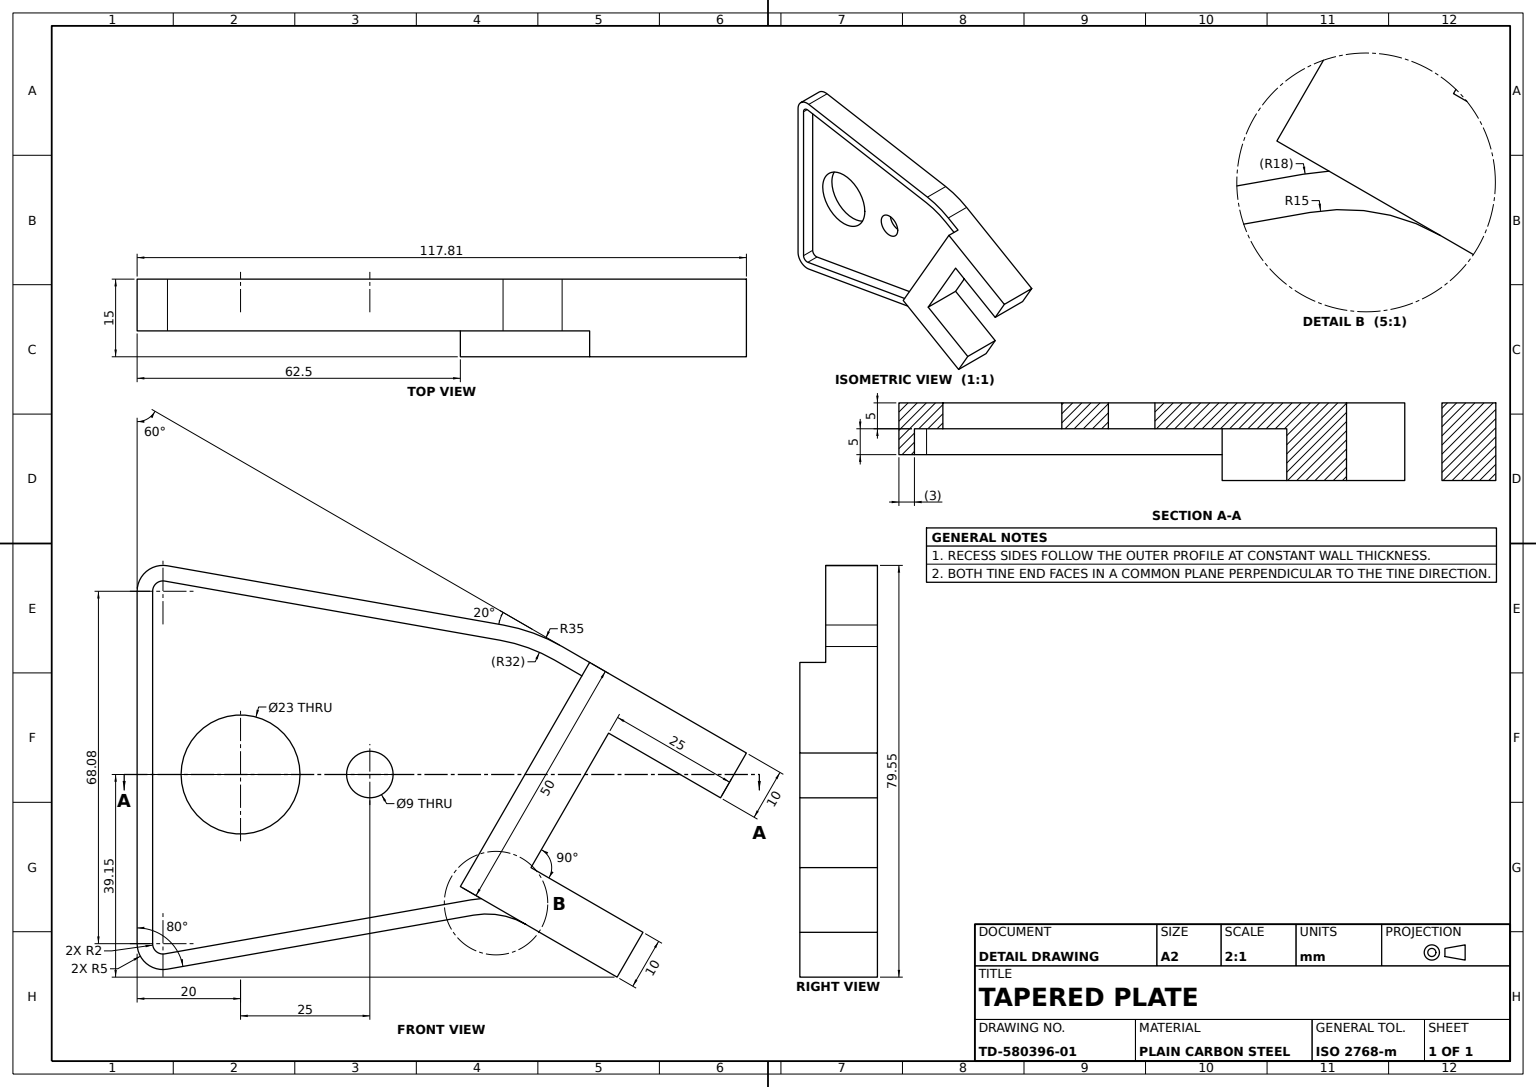
from build123d import *

# Parameters (mm, degrees)
BASE_PLATE_DEPTH    = 10
RIM_WALL_SKETCH_R   = 11.5
RIM_WALL_SKETCH_R_2 = 4.5
RIM_WALL_DEPTH      = 5
FORK_BLOCK_DEPTH    = 15


with BuildPart() as part:
    # Base Plate Profile Sketch → Base Plate (new body)
    with BuildSketch(Plane(origin=(0, 0, 0), x_dir=(1, 0, 0), z_dir=(0, 1, 0))):
        with BuildLine():
            ThreePointArc((-24.722478982, 82.179410314), (-27.300831577, 76.65011533), (-28.879861205, 70.757096532))
            Line((-28.879861205, 70.757096532), (-40.321517202, 5.868240888))
            ThreePointArc((-40.321517202, 5.868240888), (-39.227700653, 1.786061952), (-35.397478437, 0))
            Line((-35.397478437, 0), (32.684985637, 0))
            ThreePointArc((32.684985637, 0), (36.515207852, 1.786061952), (37.609024402, 5.868240888))
            Line((37.609024402, 5.868240888), (27.174016631, 65.048110745))
            ThreePointArc((27.174016631, 65.048110745), (27.174016631, 70.257556075), (28.95575187, 75.15283341))
            Line((28.95575187, 75.15283341), (23.980814684, 66.53598944))
            ThreePointArc((23.980814684, 66.53598944), (24.071961031, 65.528220723), (24.219593372, 64.527166212))
            Line((24.219593372, 64.527166212), (34.654601143, 5.347296355))
            ThreePointArc((34.654601143, 5.347296355), (34.217074523, 3.714424781), (32.684985637, 3))
            Line((32.684985637, 3), (-35.397478437, 3))
            ThreePointArc((-35.397478437, 3), (-36.929567324, 3.714424781), (-37.367093943, 5.347296355))
            Line((-37.367093943, 5.347296355), (-25.925437946, 70.236151999))
            ThreePointArc((-25.925437946, 70.236151999), (-24.481753715, 75.6240549), (-22.124402771, 80.679410314))
            Line((-22.124402771, 80.679410314), (-19.052558883, 86))
            Line((-19.052558883, 86), (-21.650635095, 87.5))
            Line((-21.650635095, 87.5), (-24.722478982, 82.179410314))
        make_face()
    extrude(amount=BASE_PLATE_DEPTH)

    # Rim Wall Sketch → Rim Wall (add)
    with BuildSketch(Plane(origin=(0, 0, 0), x_dir=(1, 0, 0), z_dir=(0, 1, 0))):
        with BuildLine():
            Line((21.650635095, 62.5), (-19.052558883, 86))
            Line((-19.052558883, 86), (-22.124402771, 80.679410314))
            ThreePointArc((-22.124402771, 80.679410314), (-24.481753715, 75.6240549), (-25.925437946, 70.236151999))
            Line((-25.925437946, 70.236151999), (-37.367093943, 5.347296355))
            ThreePointArc((-37.367093943, 5.347296355), (-36.929567324, 3.714424781), (-35.397478437, 3))
            Line((-35.397478437, 3), (32.684985637, 3))
            ThreePointArc((32.684985637, 3), (34.217074523, 3.714424781), (34.654601143, 5.347296355))
            Line((34.654601143, 5.347296355), (24.219593372, 64.527166212))
            ThreePointArc((24.219593372, 64.527166212), (24.071961031, 65.528220723), (23.980814684, 66.53598944))
            Line((23.980814684, 66.53598944), (21.650635095, 62.5))
        make_face()
        with Locations(Location((0, 20, 0), (0, 0, 270))):
            Circle(RIM_WALL_SKETCH_R, mode=Mode.SUBTRACT)
        with Locations(Location((0, 45, 0), (0, 0, 270))):
            Circle(RIM_WALL_SKETCH_R_2, mode=Mode.SUBTRACT)
    extrude(amount=RIM_WALL_DEPTH)

    # Fork Block Sketch → Fork Block (add)
    with BuildSketch(Plane(origin=(0, 0, 0), x_dir=(1, 0, 0), z_dir=(0, 1, 0))):
        Polygon((39.150635095, 92.810889132), (30.490381057, 97.810889132), (17.990381057, 76.160254038), (-7.990381057, 91.160254038), (4.509618943, 112.810889132), (-4.150635095, 117.810889132), (-21.650635095, 87.5), (21.650635095, 62.5), align=None)
    extrude(amount=FORK_BLOCK_DEPTH)


solid = part.part
